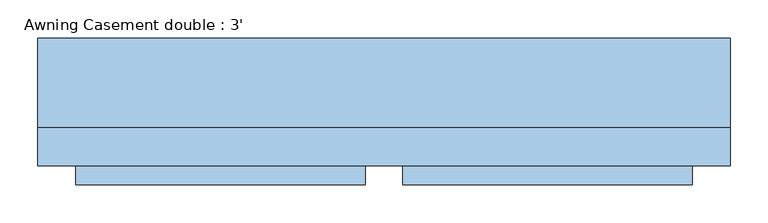
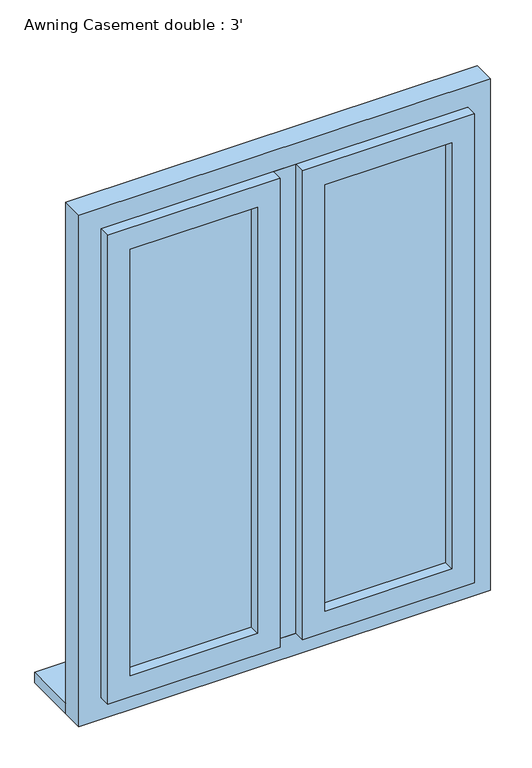
"""IFC4 building model written with IfcOpenShell, lengths in millimetres: window geometry, Awning Casement double : 3'."""

from ifc_helpers import new_model, si_unit, frame, origin, place, context, project, spatial, polyline, outline, extrude, source, transform, mapped, element, save


def awning_casement_double_3_b8244aec(model_context):
    return source(origin(), model_context, "Body", "SweptSolid", [
        extrude(outline(polyline([(2000.0, 457.2), (2000.0, -457.2), (800.0, -457.2), (800.0, 457.2), (2000.0, 457.2)]), holes=[polyline([(1950.0, 407.2), (850.0, 407.2), (850.0, -407.2), (1950.0, -407.2), (1950.0, 407.2)])]), frame((0.0, -24.5, 0.0), z_axis=(0.0, 1.0, 0.0), x_axis=(0.0, 0.0, 1.0)), (0.0, 0.0, 1.0), 50.0),
        extrude(outline(polyline([(1950.0, -25.0), (1950.0, -407.2), (850.0, -407.2), (850.0, -25.0), (1950.0, -25.0)]), holes=[polyline([(1900.0, -75.0), (900.0, -75.0), (900.0, -357.2), (1900.0, -357.2), (1900.0, -75.0)])]), frame((0.0, -49.5, 0.0), z_axis=(0.0, 1.0, 0.0), x_axis=(0.0, 0.0, 1.0)), (0.0, 0.0, 1.0), 49.5),
        extrude(outline(polyline([(1950.0, 407.2), (1950.0, 25.0), (850.0, 25.0), (850.0, 407.2), (1950.0, 407.2)]), holes=[polyline([(1900.0, 357.2), (900.0, 357.2), (900.0, 75.0), (1900.0, 75.0), (1900.0, 357.2)])]), frame((0.0, -49.5, 0.0), z_axis=(0.0, 1.0, 0.0), x_axis=(0.0, 0.0, 1.0)), (0.0, 0.0, 1.0), 49.5),
        extrude(outline(polyline([(25.0, -24.5), (-25.0, -24.5), (-25.0, 25.5), (25.0, 25.5), (25.0, -24.5)])), frame((0.0, 0.0, 850.0), z_axis=(0.0, 0.0, 1.0), x_axis=(1.0, 0.0, 0.0)), (0.0, 0.0, 1.0), 1100.0),
        extrude(outline(polyline([(-75.0, -25.5), (-357.2, -25.5), (-357.2, -24.5), (-75.0, -24.5), (-75.0, -25.5)])), frame((0.0, 0.0, 900.0), z_axis=(0.0, 0.0, 1.0), x_axis=(1.0, 0.0, 0.0)), (0.0, 0.0, 1.0), 1000.0),
        extrude(outline(polyline([(357.2, -25.5), (75.0, -25.5), (75.0, -24.5), (357.2, -24.5), (357.2, -25.5)])), frame((0.0, 0.0, 900.0), z_axis=(0.0, 0.0, 1.0), x_axis=(1.0, 0.0, 0.0)), (0.0, 0.0, 1.0), 1000.0),
        extrude(outline(polyline([(457.2, 25.5), (-457.2, 25.5), (-457.2, 144.3), (457.2, 144.3), (457.2, 25.5)])), frame((0.0, 0.0, 800.0), z_axis=(0.0, 0.0, 1.0), x_axis=(1.0, 0.0, 0.0)), (0.0, 0.0, 1.0), 25.0),
    ])


if __name__ == "__main__":
    model = new_model("IFC4")
    model_context = context("Model", 3, world=origin())
    ifc_project = project(units=[si_unit("LENGTHUNIT", "METRE", prefix="MILLI")], contexts=[model_context])
    site = spatial("IfcSite", under=ifc_project)
    building = spatial("IfcBuilding", under=site)
    placement = place(None, origin())
    awning_casement_double_3_shape = awning_casement_double_3_b8244aec(model_context)
    element("IfcWindow", 1, ObjectType="Awning Casement double : 3'", at=placement, inside=building, context=model_context, shape_type="MappedRepresentation", body=[
        mapped(awning_casement_double_3_shape, transform((0.0, 0.0, 0.0), x_axis=(1.0, 0.0, 0.0), y_axis=(0.0, 1.0, 0.0), z_axis=(0.0, 0.0, 1.0))),
    ])
    save(model, "model.ifc")

# Revit data of these elements
# Type "Awning Casement double : 3'"
#   Type Mark = "23"
#   Operation = "DoublePanelVertical"
#   Keynote = "L10/210"
#   Height = 3' - 11.24409"
#   Default Sill Height = 2' - 7.49606"
#   Width = 3' - 0"
#   Wall Closure = (empty or 0)
# Element 1 (IfcWindow, "Awning Casement double : 3'")
#   Materials on its faces: "Default Frame", "Glass", "Default Sill"
# Materials
#   "Default Frame": colour RGB 193 168 117, transparency 0
#   "Glass": class "Glass", colour RGB 0 128 192, transparency 0.75, Description = "Soda Lime Glass", Cost = 0
#   "Default Sill": colour RGB 188 165 158, transparency 0
